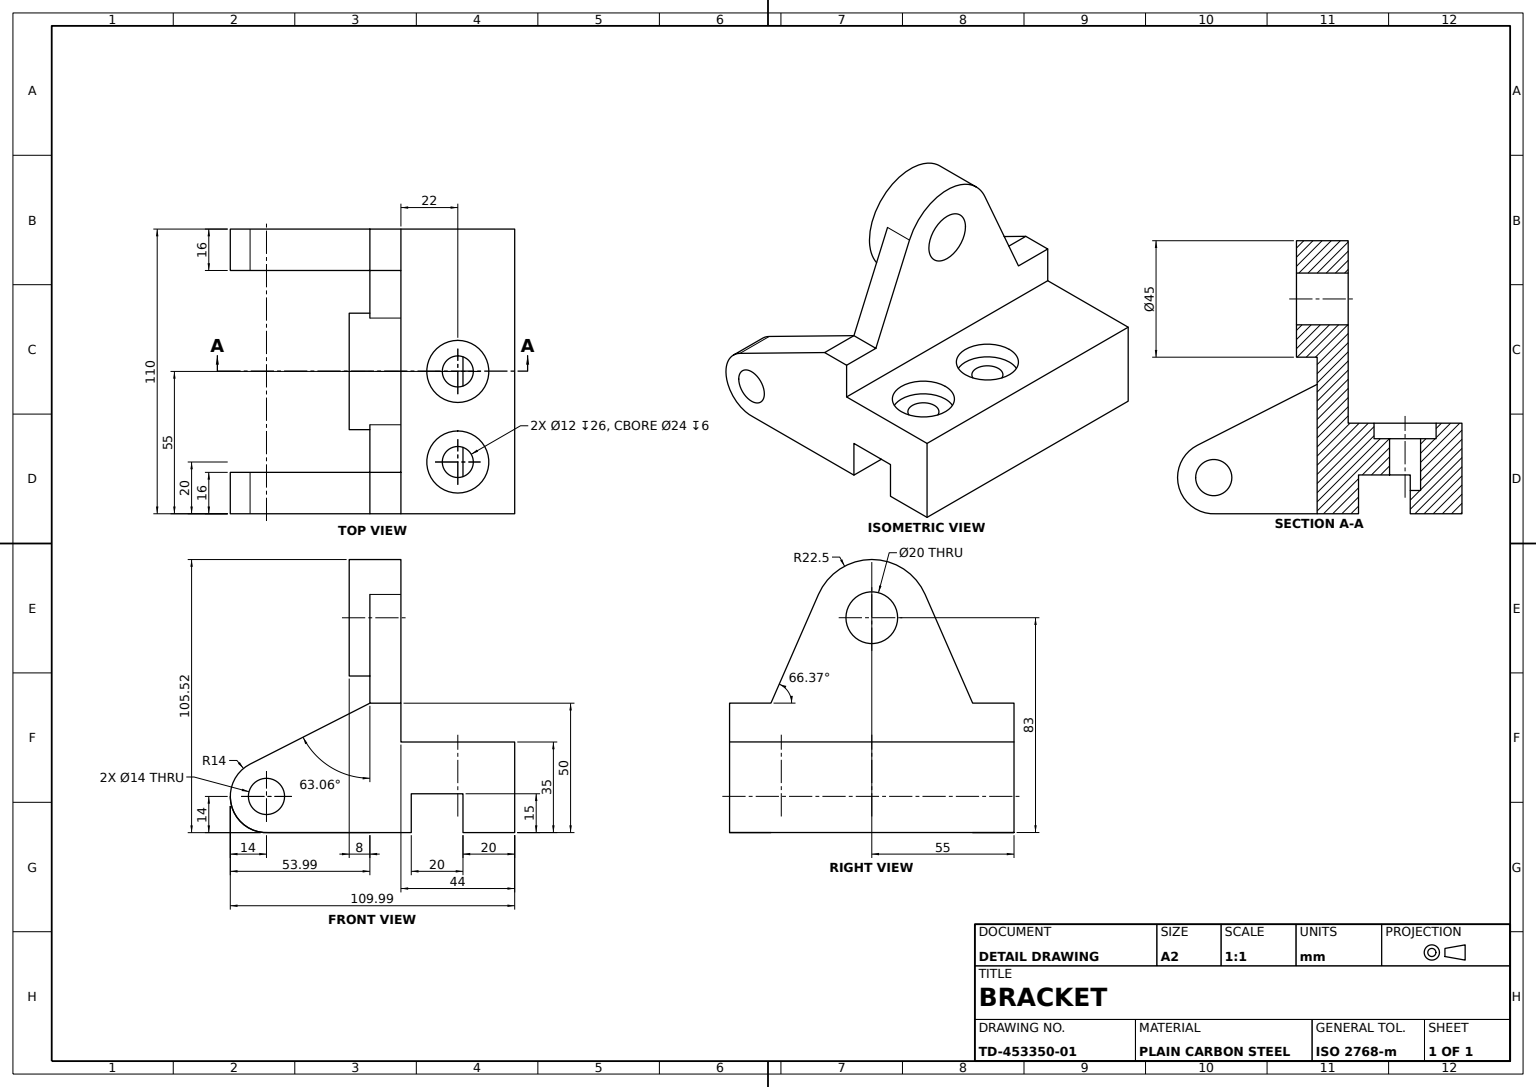
SolidWorks part; units mm, degrees
material "Plain Carbon Steel"
ref_plane "Front Plane" through (0, 0, 0) normal (0, 0, 1) x (1, 0, 0)
ref_plane "Top Plane" through (0, 0, 0) normal (0, 1, 0) x (1, 0, 0)
ref_plane "Right Plane" through (0, 0, 0) normal (1, 0, 0) x (0, 0, -1)
sketch "Base Block Sketch" plane through (0, 0, 0) normal (0, 0, 1) x (1, 0, 0)
  line L1 (50, 0) -> (50, 35)
  line L5 (-6, 35) -> (-6, 0)
  line L7 (-6, 35) -> (50, 35)
  line L8 (-6, 0) -> (50, 0)
  dimension "D1" = 56
  dimension "D2" = 35
  dimension "D3" = 6
extrude "Base Block" add sketch "Base Block Sketch" along normal blind 110
sketch "Bottom Slot Sketch" plane through (0, 0, 110) normal (0, 0, 1) x (1, 0, 0)
  line L0 (50, 0) -> (30, 0)
  line L1 (-6, 0) -> (50, 0) construction
  line L2 (30, 0) -> (10, 0)
  line L3 (10, 0) -> (10, 15)
  line L4 (10, 15) -> (30, 15)
  line L5 (30, 15) -> (30, 0)
  line L6 (10, 0) -> (30, 0)
  line L7 (50, 0) -> (50, 35) construction
  line M1 (-6, 0) -> (50, 0)
  dimension "D1" = 20
  dimension "D2" = 15
extrude "Bottom Slot" cut sketch "Bottom Slot Sketch" against normal blind 110 contours L5 L4 L3 M1
sketch "Side Step Sketch" plane through (0, 0, 110) normal (0, 0, 1) x (1, 0, 0)
  line L0 (-6, 35) -> (6, 35)
  line L1 (50, 35) -> (-6, 35) construction
  line L2 (6, 35) -> (6, 50)
  line L3 (6, 50) -> (-6, 50)
  line L4 (-6, 50) -> (-6, 35)
  line L5 (50, 0) -> (50, 35) construction
  line L6 (30, 0) -> (50, 0) construction
  dimension "D1" = 44
  dimension "D2" = 50
extrude "Side Step" add sketch "Side Step Sketch" against normal blind 110
sketch "Side Lug 1 Sketch" plane through (0, 0, 110) normal (0, 0, 1) x (1, 0, 0)
  line L0 (-6, 0) -> (-45.9873, 0)
  line L1 (-6, 50) -> (-6, 0)
  line L2 (-6, 50) -> (-52.3299, 26.4559)
  line L3 (50, 0) -> (50, 35) construction
  arc A0 (-52.3299, 26.4559) -> (-45.1511, 0) centre (-45.9873, 13.975) ccw
  dimension "D1" = 14
  dimension "D2" = 95.1511
  dimension "D3" = 95.9873
extrude "Side Lug 1" add sketch "Side Lug 1 Sketch" against normal blind 16
sketch "Side Hole 1 Sketch" plane through (0, 0, 110) normal (0, 0, 1) x (1, 0, 0)
  circle A0 centre (-45.9873, 13.975) radius 7
  dimension "D1" = 14
extrude "Side Hole 1" cut sketch "Side Hole 1 Sketch" against normal blind 16
sketch "Side Lug 2 Sketch" plane through (0, 0, 0) normal (0, 0, -1) x (-1, 0, 0)
  line L0 (6, 50) -> (6, 0)
  line L1 (6, 0) -> (45.1511, 0)
  line L2 (6, 50) -> (52.3299, 26.4559)
  arc A0 (45.1511, 0) -> (52.3299, 26.4559) centre (45.9873, 13.975) ccw
extrude "Side Lug 2" add sketch "Side Lug 2 Sketch" against normal blind 16
sketch "Side Hole 2 Sketch" plane through (0, 0, 0) normal (0, 0, -1) x (-1, 0, 0)
  circle A0 centre (45.9873, 13.975) radius 7
  dimension "D1" = 14
extrude "Side Hole 2" cut sketch "Side Hole 2 Sketch" against normal blind 16
sketch "Upright Ear Sketch" plane through (-6, 0, 0) normal (-1, 0, 0) x (0, 0, 1)
  line L2 (34.3871, 92.0198) -> (16, 50)
  line L3 (16, 50) -> (94, 50)
  line L4 (94, 50) -> (75.6129, 92.0198)
  arc A0 (75.6129, 92.0198) -> (34.3871, 92.0198) centre (55, 83) ccw
  dimension "D1" = 45
  dimension "D2" = 22.5
  dimension "D3" = 18.3871
extrude "Upright Ear" add sketch "Upright Ear Sketch" against normal blind 12
sketch "Pivot Boss Ø45 Sketch" plane through (-6, 0, 0) normal (-1, 0, 0) x (0, 0, 1)
  circle A0 centre (55, 83) radius 22.5
  dimension "D1" = 45
  dimension "D2" = 45
extrude "Pivot Boss Ø45" add sketch "Pivot Boss Ø45 Sketch" along normal blind 8
sketch "Pivot Bore Ø20 Sketch" plane through (-14, 0, 0) normal (-1, 0, 0) x (0, 0, 1)
  circle A0 centre (55, 83) radius 10
  dimension "D1" = 20
  dimension "D2" = 20
extrude "Pivot Bore Ø20" cut sketch "Pivot Bore Ø20 Sketch" against normal blind 20
sketch "Counterbores 2xØ24 Sketch" plane through (0, 35, 0) normal (0, 1, 0) x (1, 0, 0)
  line L0 (6, 0) -> (6, -110) construction
  line L1 (50, 0) -> (6, 0) construction
  circle A0 centre (28, -90) radius 12
  circle A1 centre (28, -55) radius 12
  dimension "D1" = 24
  dimension "D2" = 24
  dimension "D3" = 24
  dimension "D4" = 22
  dimension "D5" = 55
  dimension "D6" = 90
extrude "Counterbores 2xØ24" cut sketch "Counterbores 2xØ24 Sketch" against normal blind 6
sketch "Holes 2xØ12 Sketch" plane through (0, 29, 0) normal (0, 1, 0) x (1, 0, 0)
  circle A0 centre (28, -55) radius 6
  circle A1 centre (28, -90) radius 6
  dimension "D1" = 12
  dimension "D2" = 12
  dimension "D3" = 12
extrude "Holes 2xØ12" cut sketch "Holes 2xØ12 Sketch" against normal blind 20
